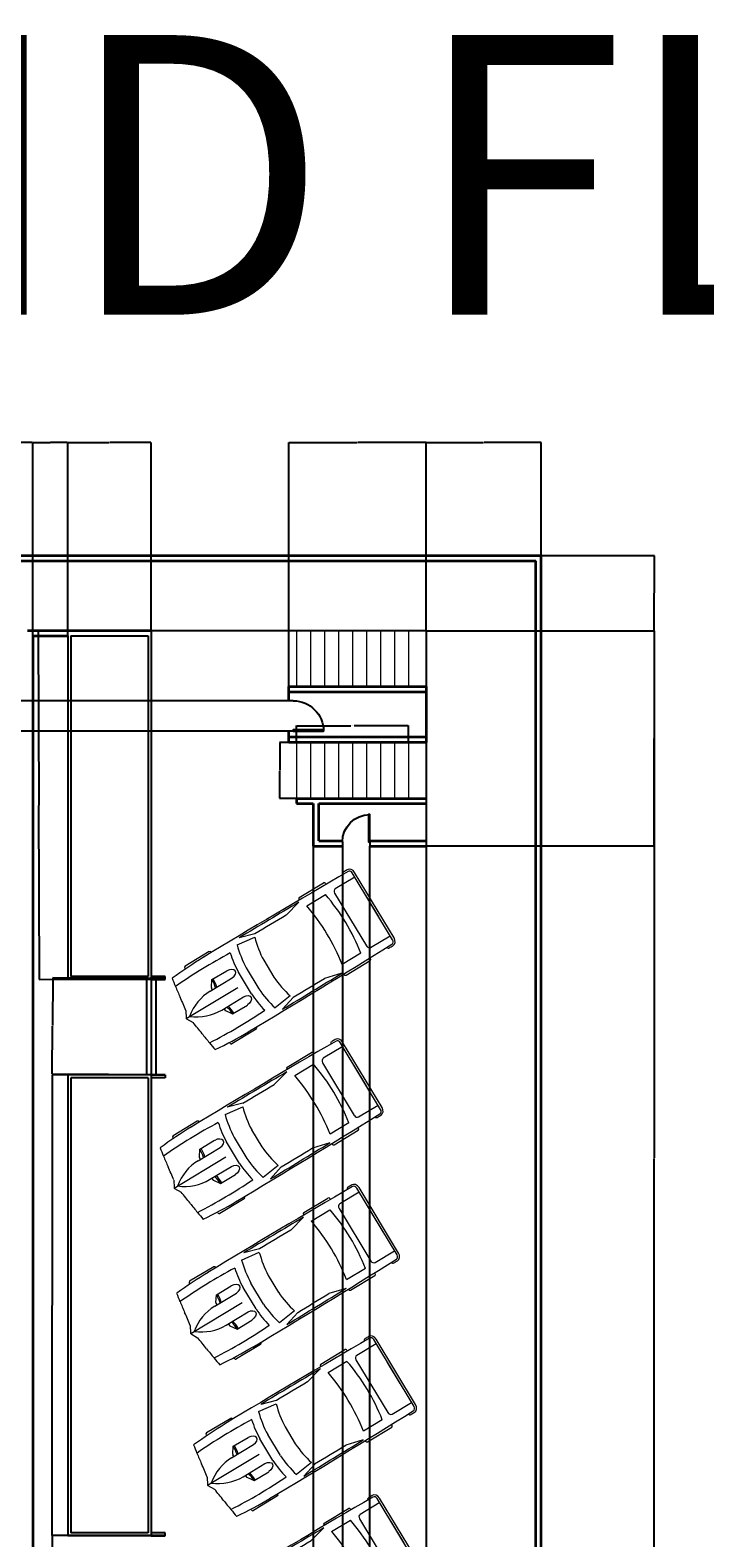
# Model space of a CAD drawing. Units: inches. Extents: x 1563 to 5866, y -225 to 2207.
# Tile 3 of 3: x 3624 to 4202, y 913 to 2207. Entities that reach past the tile are written whole.
import ezdxf

# ---------------------------------------------------------------- set-up
doc = ezdxf.new("R2010")
doc.units = ezdxf.units.IN
for name, color, linetype, lineweight in [('A-ANNO-DIMS', 2, 'Continuous', 18), ('A-ANNO-TEXT', 7, 'Continuous', 25), ('A-DOOR', 4, 'Continuous', 25), ('A-FLOR-STRS', 3, 'Continuous', 18), ('A-WALL', 7, 'Continuous', 35), ('C-PKNG', 8, 'Continuous', 25), ('C-PKNG-VEHI', 9, 'Continuous', 13), ('C-PROP', 2, 'Continuous', 35)]:
    doc.layers.add(name, color=color, linetype=linetype, lineweight=lineweight)
doc.styles.get("Standard").update_dxf_attribs({"font": 'arial.ttf'})
doc.dimstyles.get("Standard").update_dxf_attribs({"dimtxt": 0.18, "dimasz": 0.18, "dimexe": 0.18, "dimexo": 0.0625, "dimgap": 0.09, "dimtad": 0, "dimtih": 1, "dimtoh": 1, "dimdec": 4, "dimzin": 0, "dimdsep": 46, "dimtxsty": 'Standard', "dimcen": 0.09, "dimadec": 0, "dimazin": 0, "dimtfac": 1, "dimtdec": 4, "dimtofl": 0, "dimtmove": 0, "dimatfit": 3, "dimfxl": 1, "dimtolj": 1, "dimtzin": 0, "dimarcsym": 0})

# ---------------------------------------------------------------- blocks, each defined once
blk = doc.blocks.new('*U2')
for p, q in [((46.6, 38.9), (22.4, 38.9)), ((136.7, 38.9), (160.9, 38.9)), ((21.1, 37.4), (21.1, 36.8)), ((47.8, 37.4), (47.8, 37.4)), ((70, 31.5), (86.4, 29.4)), ((88, 31.9), (74.8, 35.9)), ((134.3, 35.6), (119.3, 31.8)), ((135.5, 37.1), (135.5, 37.4)), ((138.4, 29.4), (157.2, 29.4)), ((162.1, 37.4), (162.1, 36.8)), ((164.5, 26.4), (164.5, -26.4)), ((186.5, 29.4), (167, 29.4)), ((186.5, -33.5), (186.5, 33.5)), ((188.4, -32.8), (188.4, 32.8)), ((32.3, 11.6), (36.1, 17.2)), ((36.1, 17.2), (50.9, 17.2)), ((3.3, 6.1), (0.1, 0.4)), ((29.8, 9.5), (51.7, 9.5)), ((32.1, 9.5), (32.1, 11.2)), ((58.9, -10.8), (58.9, 10.8)), ((66.6, -10.5), (66.6, 10.5)), ((82.7, 8.5), (82.7, -8.5)), ((186.5, -10.5), (186.5, 10.5)), ((0, 0), (51.7, 0)), ((0.1, -0.4), (3.3, -6.1)), ((29.8, -9.5), (51.7, -9.5)), ((32.1, -9.5), (32.1, -11.2)), ((32.3, -11.6), (36.1, -17.2)), ((36.1, -17.2), (50.9, -17.2)), ((21.1, -37.4), (21.1, -36.8)), ((47.8, -37.4), (47.8, -37.4)), ((86.4, -29.4), (70, -31.5)), ((88, -31.9), (74.8, -35.9)), ((134.3, -35.6), (119.3, -31.8)), ((135.5, -37.1), (135.5, -37.4)), ((157.2, -29.4), (138.4, -29.4)), ((162.1, -37.4), (162.1, -36.8)), ((167, -29.4), (186.5, -29.4)), ((46.6, -38.9), (22.4, -38.9)), ((136.7, -38.9), (160.9, -38.9))]:
    blk.add_line(p, q)
for centre, major_axis, ratio, start_param, end_param in [((22.4, 37.4), (0, -1.48), 0.842304, 3.141593, 4.712389), ((46.6, 37.4), (0, 1.48), 0.842304, -1.570796, 0), ((136.7, 37.4), (0, -1.48), 0.842304, 3.141593, 4.712389), ((160.9, 37.4), (0, 1.48), 0.842304, -1.570796, 0), ((259.2, -27.5), (0, -305.3), 0.842304, 4.528606, 4.561838), ((266, -27.5), (0, 313.3), 0.842304, 1.367076, 1.39176), ((37.5, -594), (0, -623.3), 0.842304, 3.096046, 3.200911), ((41.2, -490.9), (0, 528.2), 0.842304, 0.00281, 0.075598), ((64.5, -10555.6), (0, 10593), 0.842304, -0.013397, 0.002797), ((134.4, 5.4), (0, -89.8), 0.842304, 4.449482, 4.652344), ((135.3, 5.4), (0, 81.8), 0.842304, 1.245306, 1.50788), ((64.5, -10555.6), (0, -10591.5), 0.842304, 3.133765, 3.140441), ((149.6, 2.8), (0, -79.6), 0.842304, 4.372215, 4.640744), ((95.8, -3666.4), (0, -3698.2), 0.842304, 3.134049, 3.144098), ((17.1, 0), (0, 147), 0.842304, 4.511394, 4.913384), ((35.9, 0), (0, 147), 0.842304, 4.511394, 4.913384), ((167, 26.4), (0, 2.96), 0.842304, 0, 1.570796), ((180.6, 35.8), (0, 2.22), 0.842304, -0.013017, 1.249894), ((64.5, -10556.4), (0, 10595.3), 0.842304, -0.013397, -0.013017), ((184, 32.8), (0, -5.25), 0.842304, 1.570796, 3.128196), ((184, 33.5), (0, -2.96), 0.842304, 1.570796, 3.128196), ((-204.5, 52.4), (0, -251), 0.842304, 1.385369, 1.434372), ((13, 17), (0, 27.4), 0.842304, 4.435146, 4.718221), ((14.2, 17), (0, 27.4), 0.842304, 4.435146, 4.718221), ((50.8, 13.3), (6.34, -0.36), 0.603834, -1.395552, 1.581315), ((0.6, 0), (0, -0.74), 0.842304, 4.131459, 5.293319), ((29.8, -46.7), (0, 56.2), 0.842304, 0, 0.590319), ((32.7, 11.2), (0, 0.74), 0.842304, 0.879714, 1.570796), ((-204.5, -52.4), (0, 251), 0.842304, -1.434372, -1.385369), ((29.8, 46.7), (0, 56.2), 0.842304, 2.551274, 3.141593), ((32.7, -11.2), (0, -0.74), 0.842304, 4.712389, 5.403472), ((13, -17), (0, -27.4), 0.842304, 1.564964, 1.848039), ((14.2, -17), (0, -27.4), 0.842304, 1.564964, 1.848039), ((134.4, -5.4), (0, -89.8), 0.842304, -1.510751, -1.307889), ((135.3, -5.4), (0, -81.8), 0.842304, -1.50788, -1.245306), ((149.6, -2.8), (0, -79.6), 0.842304, -1.499151, -1.230623), ((259.2, 27.5), (0, 305.3), 0.842304, 1.721348, 1.754579), ((266, 27.5), (0, 313.3), 0.842304, 1.749832, 1.774517), ((37.5, 594), (0, -623.3), 0.842304, -0.059319, 0.045547), ((41.2, 490.9), (0, -528.2), 0.842304, -0.075598, -0.00281), ((22.4, -37.4), (0, 1.48), 0.842304, 1.570796, 3.141593), ((64.5, 10555.6), (0, 10593), 0.842304, 3.138796, 3.15499), ((46.6, -37.4), (0, -1.48), 0.842304, 0, 1.570796), ((64.5, 10555.6), (0, -10591.5), 0.842304, 0.001152, 0.007828), ((95.8, 3666.4), (0, -3698.2), 0.842304, -0.002505, 0.007544), ((136.7, -37.4), (0, -1.48), 0.842304, -1.570796, 0), ((160.9, -37.4), (0, 1.48), 0.842304, 3.141593, 4.712389), ((167, -26.4), (0, -2.96), 0.842304, 4.712389, 6.283185), ((180.6, -35.8), (0, -2.22), 0.842304, -1.249894, 0.013017), ((64.5, 10556.4), (0, 10595.3), 0.842304, 3.15461, 3.15499), ((184, -32.8), (0, -5.25), 0.842304, 0.013397, 1.570796), ((184, -33.5), (0, 2.96), 0.842304, 3.15499, 4.712389)]:
    blk.add_ellipse(centre, major_axis=major_axis, ratio=ratio, start_param=start_param, end_param=end_param)
at = {"extrusion": (0, 0, -1)}
blk.add_ellipse((50.8, -13.3), major_axis=(6.34, 0.36), ratio=0.603834, start_param=-1.395552, end_param=1.581315, dxfattribs=at)
blk = doc.blocks.new('*U5')
for p, q in [((0, 0), (0, -6)), ((40, 0), (40, -6))]:
    blk.add_line(p, q)
blk.add_lwpolyline([(0, 0), (0, 40), (1.75, 40), (1.75, 0)], close=True)
blk.add_arc((0, 0), 40, 0, 90)
blk = doc.blocks.new('STAIR-FLIGHT-48IN')
for p, q in [((0, 48), (0, 0)), ((12, 48), (12, 0)), ((24, 48), (24, 0)), ((36, 48), (36, 0)), ((48, 48), (48, 0)), ((60, 48), (60, 0)), ((72, 48), (72, 0)), ((84, 48), (84, 0)), ((96, 48), (96, 0))]:
    blk.add_line(p, q)
blk = doc.blocks.new('*D16')
at = {"layer": 'A-ANNO-DIMS', "color": 0, "lineweight": -2, "transparency": 16777216}
for p, q in [((3852.2, 1595.9), (3852.2, 1610.4)), ((3852.4, 1610.2), (3898.8, 1610.2)), ((3948, 1610.2), (3901.6, 1610.2)), ((3948.2, 1595.9), (3948.2, 1610.4))]:
    blk.add_line(p, q, dxfattribs=at)
at = {"layer": 'A-ANNO-DIMS', "color": 0, "transparency": 16777216}
for points in [[(3852.4, 1610.2), (3852.4, 1610.2), (3852.2, 1610.2)], [(3948, 1610.2), (3948, 1610.2), (3948.2, 1610.2)]]:
    blk.add_solid(points, dxfattribs=at)
at = {"layer": 'Defpoints', "color": 0, "transparency": 16777216}
for p in [(3948.2, 1610.2), (3852.2, 1595.8), (3948.2, 1595.8)]:
    blk.add_point(p, dxfattribs=at)
at = {"layer": 'A-ANNO-DIMS', "color": 0, "transparency": 16777216, "insert": (3900.2, 1610.2), "char_height": 0.18, "attachment_point": 5}
blk.add_mtext('\\A1;STAIR FLIGHT 96 TYP.', dxfattribs=at)
blk = doc.blocks.new('*D17')
at = {"layer": 'A-ANNO-DIMS', "color": 0, "lineweight": -2, "transparency": 16777216}
for p, q in [((3852.1, 1595.8), (3837.6, 1595.8)), ((3837.8, 1595.6), (3837.8, 1572)), ((3837.8, 1548), (3837.8, 1571.6)), ((3852.1, 1547.8), (3837.6, 1547.8))]:
    blk.add_line(p, q, dxfattribs=at)
at = {"layer": 'A-ANNO-DIMS', "color": 0, "transparency": 16777216}
for points in [[(3837.8, 1595.6), (3837.8, 1595.6), (3837.8, 1595.8)], [(3837.8, 1548), (3837.8, 1548), (3837.8, 1547.8)]]:
    blk.add_solid(points, dxfattribs=at)
at = {"layer": 'Defpoints', "color": 0, "transparency": 16777216}
for p in [(3837.8, 1595.8), (3852.2, 1595.8), (3852.2, 1547.8)]:
    blk.add_point(p, dxfattribs=at)
at = {"layer": 'A-ANNO-DIMS', "color": 0, "transparency": 16777216, "insert": (3837.8, 1571.8), "char_height": 0.18, "attachment_point": 5}
blk.add_mtext('\\A1;48 TYP.', dxfattribs=at)
blk = doc.blocks.new('*D20')
at = {"layer": 'A-ANNO-DIMS', "color": 0, "lineweight": -2, "transparency": 16777216}
for p, q in [((3379.6, 1756.4), (3379.6, 1853.4)), ((3379.8, 1853.2), (3502.4, 1853.2)), ((3625.8, 1853.2), (3503.2, 1853.2)), ((3626, 1687.4), (3626, 1853.4))]:
    blk.add_line(p, q, dxfattribs=at)
at = {"layer": 'A-ANNO-DIMS', "color": 0, "transparency": 16777216}
for points in [[(3379.8, 1853.2), (3379.8, 1853.2), (3379.6, 1853.2)], [(3625.8, 1853.2), (3625.8, 1853.2), (3626, 1853.2)]]:
    blk.add_solid(points, dxfattribs=at)
at = {"layer": 'Defpoints', "color": 0, "transparency": 16777216}
for p in [(3626, 1853.2), (3379.6, 1756.3), (3626, 1687.3)]:
    blk.add_point(p, dxfattribs=at)
at = {"layer": 'A-ANNO-DIMS', "color": 0, "transparency": 16777216, "insert": (3502.8, 1853.2), "char_height": 0.18, "attachment_point": 5}
blk.add_mtext('\\A1;246.4', dxfattribs=at)
blk = doc.blocks.new('*D21')
at = {"layer": 'A-ANNO-DIMS', "color": 0, "lineweight": -2, "transparency": 16777216}
for p, q in [((3626, 1687.4), (3626, 1853.4)), ((3626.2, 1853.2), (3640.8, 1853.2)), ((3655.8, 1853.2), (3641.2, 1853.2)), ((3656, 1687.4), (3656, 1853.4))]:
    blk.add_line(p, q, dxfattribs=at)
at = {"layer": 'A-ANNO-DIMS', "color": 0, "transparency": 16777216}
for points in [[(3626.2, 1853.2), (3626.2, 1853.2), (3626, 1853.2)], [(3655.8, 1853.2), (3655.8, 1853.2), (3656, 1853.2)]]:
    blk.add_solid(points, dxfattribs=at)
at = {"layer": 'Defpoints', "color": 0, "transparency": 16777216}
for p in [(3656, 1853.2), (3626, 1687.3), (3656, 1687.3)]:
    blk.add_point(p, dxfattribs=at)
at = {"layer": 'A-ANNO-DIMS', "color": 0, "transparency": 16777216, "insert": (3641, 1853.2), "char_height": 0.18, "attachment_point": 5}
blk.add_mtext('\\A1;30', dxfattribs=at)
blk = doc.blocks.new('*D22')
at = {"layer": 'A-ANNO-DIMS', "color": 0, "lineweight": -2, "transparency": 16777216}
for p, q in [((3656, 1687.4), (3656, 1853.4)), ((3656.2, 1853.2), (3691.4, 1853.2)), ((3727.3, 1853.2), (3692.1, 1853.2)), ((3727.5, 1691.9), (3727.5, 1853.4))]:
    blk.add_line(p, q, dxfattribs=at)
at = {"layer": 'A-ANNO-DIMS', "color": 0, "transparency": 16777216}
for points in [[(3656.2, 1853.2), (3656.2, 1853.2), (3656, 1853.2)], [(3727.3, 1853.2), (3727.3, 1853.2), (3727.5, 1853.2)]]:
    blk.add_solid(points, dxfattribs=at)
at = {"layer": 'Defpoints', "color": 0, "transparency": 16777216}
for p in [(3727.5, 1853.2), (3656, 1687.3), (3727.5, 1691.8)]:
    blk.add_point(p, dxfattribs=at)
at = {"layer": 'A-ANNO-DIMS', "color": 0, "transparency": 16777216, "insert": (3691.7, 1853.2), "char_height": 0.18, "attachment_point": 5}
blk.add_mtext('\\A1;71.5', dxfattribs=at)
blk = doc.blocks.new('*D24')
at = {"layer": 'A-ANNO-DIMS', "color": 0, "lineweight": -2, "transparency": 16777216}
for p, q in [((3963.5, 1691.9), (3963.5, 1853.4)), ((3963.7, 1853.2), (4012.4, 1853.2)), ((4061.9, 1853.2), (4013.2, 1853.2)), ((4062.1, 1756.4), (4062.1, 1853.4))]:
    blk.add_line(p, q, dxfattribs=at)
at = {"layer": 'A-ANNO-DIMS', "color": 0, "transparency": 16777216}
for points in [[(3963.7, 1853.2), (3963.7, 1853.2), (3963.5, 1853.2)], [(4061.9, 1853.2), (4061.9, 1853.2), (4062.1, 1853.2)]]:
    blk.add_solid(points, dxfattribs=at)
at = {"layer": 'Defpoints', "color": 0, "transparency": 16777216}
for p in [(4062.1, 1853.2), (4062.1, 1756.3), (3963.5, 1691.8)]:
    blk.add_point(p, dxfattribs=at)
at = {"layer": 'A-ANNO-DIMS', "color": 0, "transparency": 16777216, "insert": (4012.8, 1853.2), "char_height": 0.18, "attachment_point": 5}
blk.add_mtext('\\A1;98.58', dxfattribs=at)
blk = doc.blocks.new('*D25')
at = {"layer": 'A-ANNO-DIMS', "color": 0, "lineweight": -2, "transparency": 16777216}
for p, q in [((4062.1, 1756.3), (4159.1, 1756.3)), ((4159, 1756.1), (4159, 1724.2)), ((4159, 1692), (4159, 1723.9)), ((3963.5, 1691.8), (4159.1, 1691.8))]:
    blk.add_line(p, q, dxfattribs=at)
at = {"layer": 'A-ANNO-DIMS', "color": 0, "transparency": 16777216}
for points in [[(4158.9, 1756.1), (4159, 1756.1), (4159, 1756.3)], [(4158.9, 1692), (4159, 1692), (4159, 1691.8)]]:
    blk.add_solid(points, dxfattribs=at)
at = {"layer": 'Defpoints', "color": 0, "transparency": 16777216}
for p in [(4062.1, 1756.3), (4159, 1756.3), (3963.5, 1691.8)]:
    blk.add_point(p, dxfattribs=at)
at = {"layer": 'A-ANNO-DIMS', "color": 0, "transparency": 16777216, "insert": (4159, 1724.1), "char_height": 0.18, "attachment_point": 5}
blk.add_mtext('\\A1;64.5', dxfattribs=at)
blk = doc.blocks.new('*D26')
at = {"layer": 'A-ANNO-DIMS', "color": 0, "lineweight": -2, "transparency": 16777216}
for p, q in [((3963.5, 1691.8), (4159.1, 1691.8)), ((4159, 1691.6), (4159, 1599.6)), ((4159, 1507.1), (4159, 1599.2)), ((3963.5, 1507), (4159.1, 1507))]:
    blk.add_line(p, q, dxfattribs=at)
at = {"layer": 'A-ANNO-DIMS', "color": 0, "transparency": 16777216}
for points in [[(4158.9, 1691.6), (4159, 1691.6), (4159, 1691.8)], [(4158.9, 1507.1), (4159, 1507.1), (4159, 1507)]]:
    blk.add_solid(points, dxfattribs=at)
at = {"layer": 'Defpoints', "color": 0, "transparency": 16777216}
for p in [(3963.5, 1691.8), (4159, 1691.8), (3963.5, 1507)]:
    blk.add_point(p, dxfattribs=at)
at = {"layer": 'A-ANNO-DIMS', "color": 0, "transparency": 16777216, "insert": (4159, 1599.4), "char_height": 0.18, "attachment_point": 5}
blk.add_mtext('\\A1;184.86', dxfattribs=at)
blk = doc.blocks.new('*D27')
at = {"layer": 'A-ANNO-DIMS', "color": 0, "lineweight": -2, "transparency": 16777216}
for p, q in [((3963.5, 1691.8), (4159.1, 1691.8)), ((4159, 1691.6), (4159, 1239.2)), ((4159, 786.4), (4159, 1238.8)), ((3963.5, 786.2), (4159.1, 786.2))]:
    blk.add_line(p, q, dxfattribs=at)
at = {"layer": 'A-ANNO-DIMS', "color": 0, "transparency": 16777216}
for points in [[(4158.9, 1691.6), (4159, 1691.6), (4159, 1691.8)], [(4158.9, 786.4), (4159, 786.4), (4159, 786.2)]]:
    blk.add_solid(points, dxfattribs=at)
at = {"layer": 'Defpoints', "color": 0, "transparency": 16777216}
for p in [(3963.5, 1691.8), (4159, 1691.8), (3963.5, 786.2)]:
    blk.add_point(p, dxfattribs=at)
at = {"layer": 'A-ANNO-DIMS', "color": 0, "transparency": 16777216, "insert": (4159, 1239), "char_height": 0.18, "attachment_point": 5}
blk.add_mtext('\\A1;905.6', dxfattribs=at)
blk = doc.blocks.new('*D39')
at = {"layer": 'A-ANNO-DIMS', "color": 0, "lineweight": -2, "transparency": 16777216}
for p, q in [((3727.4, 1691.8), (3630.4, 1691.5)), ((3630.6, 1691.3), (3631.1, 1542)), ((3631.6, 1392.3), (3631.1, 1541.6)), ((3728.5, 1392.5), (3631.5, 1392.1))]:
    blk.add_line(p, q, dxfattribs=at)
at = {"layer": 'A-ANNO-DIMS', "color": 0, "transparency": 16777216}
for points in [[(3630.6, 1691.3), (3630.6, 1691.3), (3630.6, 1691.5)], [(3631.7, 1392.3), (3631.6, 1392.3), (3631.6, 1392.1)]]:
    blk.add_solid(points, dxfattribs=at)
at = {"layer": 'Defpoints', "color": 0, "transparency": 16777216}
for p in [(3630.6, 1691.5), (3727.5, 1691.8), (3728.5, 1392.5)]:
    blk.add_point(p, dxfattribs=at)
at = {"layer": 'A-ANNO-DIMS', "color": 0, "transparency": 16777216, "insert": (3631.1, 1541.8), "char_height": 0.18, "attachment_point": 5}
blk.add_mtext('\\A1;299.36', dxfattribs=at)
blk = doc.blocks.new('*D40')
at = {"layer": 'A-ANNO-DIMS', "color": 0, "lineweight": -2, "transparency": 16777216}
for p, q in [((3643.3, 1393.8), (3642.9, 1352.8)), ((3740.1, 1393.1), (3643.1, 1393.9)), ((3642.6, 1311.4), (3642.9, 1352.4)), ((3739.4, 1310.5), (3642.4, 1311.2))]:
    blk.add_line(p, q, dxfattribs=at)
at = {"layer": 'A-ANNO-DIMS', "color": 0, "transparency": 16777216}
for points in [[(3643.2, 1393.8), (3643.3, 1393.8), (3643.3, 1393.9)], [(3642.6, 1311.4), (3642.6, 1311.4), (3642.6, 1311.2)]]:
    blk.add_solid(points, dxfattribs=at)
at = {"layer": 'Defpoints', "color": 0, "transparency": 16777216}
for p in [(3643.3, 1393.9), (3740.2, 1393.1), (3739.5, 1310.5)]:
    blk.add_point(p, dxfattribs=at)
at = {"layer": 'A-ANNO-DIMS', "color": 0, "transparency": 16777216, "insert": (3642.9, 1352.6), "char_height": 0.18, "attachment_point": 5}
blk.add_mtext('\\A1;82.7', dxfattribs=at)
blk = doc.blocks.new('*D41')
at = {"layer": 'A-ANNO-DIMS', "color": 0, "lineweight": -2, "transparency": 16777216}
for p, q in [((3739.4, 1310.5), (3642.4, 1310.5)), ((3642.6, 1310.3), (3642.6, 1112.9)), ((3642.6, 915.1), (3642.6, 1112.5)), ((3739.4, 915), (3642.4, 915))]:
    blk.add_line(p, q, dxfattribs=at)
at = {"layer": 'A-ANNO-DIMS', "color": 0, "transparency": 16777216}
for points in [[(3642.5, 1310.3), (3642.6, 1310.3), (3642.6, 1310.5)], [(3642.5, 915.1), (3642.6, 915.1), (3642.6, 915)]]:
    blk.add_solid(points, dxfattribs=at)
at = {"layer": 'Defpoints', "color": 0, "transparency": 16777216}
for p in [(3642.6, 1310.5), (3739.5, 1310.5), (3739.5, 915)]:
    blk.add_point(p, dxfattribs=at)
at = {"layer": 'A-ANNO-DIMS', "color": 0, "transparency": 16777216, "insert": (3642.6, 1112.7), "char_height": 0.18, "attachment_point": 5}
blk.add_mtext('\\A1;395.5', dxfattribs=at)
blk = doc.blocks.new('*D42')
at = {"layer": 'A-ANNO-DIMS', "color": 0, "lineweight": -2, "transparency": 16777216}
for p, q in [((3739.4, 915), (3642.4, 915)), ((3642.6, 914.8), (3642.6, 870.8)), ((3642.6, 826.6), (3642.6, 870.5)), ((3739.4, 826.4), (3642.4, 826.4))]:
    blk.add_line(p, q, dxfattribs=at)
at = {"layer": 'A-ANNO-DIMS', "color": 0, "transparency": 16777216}
for points in [[(3642.5, 914.8), (3642.6, 914.8), (3642.6, 915)], [(3642.5, 826.6), (3642.6, 826.6), (3642.6, 826.4)]]:
    blk.add_solid(points, dxfattribs=at)
at = {"layer": 'Defpoints', "color": 0, "transparency": 16777216}
for p in [(3642.6, 915), (3739.5, 915), (3739.5, 826.4)]:
    blk.add_point(p, dxfattribs=at)
at = {"layer": 'A-ANNO-DIMS', "color": 0, "transparency": 16777216, "insert": (3642.6, 870.7), "char_height": 0.18, "attachment_point": 5}
blk.add_mtext('\\A1;88.58', dxfattribs=at)
blk = doc.blocks.new('*D44')
at = {"layer": 'A-ANNO-DIMS', "color": 0, "lineweight": -2, "transparency": 16777216}
for p, q in [((3845.4, 1631.6), (2993.3, 1631.6)), ((2993.5, 1631.4), (2993.5, 1618.8)), ((2993.5, 1605.8), (2993.5, 1618.4)), ((3845.4, 1605.6), (2993.3, 1605.6))]:
    blk.add_line(p, q, dxfattribs=at)
at = {"layer": 'A-ANNO-DIMS', "color": 0, "transparency": 16777216}
for points in [[(2993.4, 1631.4), (2993.5, 1631.4), (2993.5, 1631.6)], [(2993.4, 1605.8), (2993.5, 1605.8), (2993.5, 1605.6)]]:
    blk.add_solid(points, dxfattribs=at)
at = {"layer": 'Defpoints', "color": 0, "transparency": 16777216}
for p in [(2993.5, 1631.6), (3845.5, 1631.6), (3845.5, 1605.6)]:
    blk.add_point(p, dxfattribs=at)
at = {"layer": 'A-ANNO-DIMS', "color": 0, "transparency": 16777216, "insert": (2993.5, 1618.6), "char_height": 0.18, "attachment_point": 5}
blk.add_mtext('\\A1;25.95', dxfattribs=at)
blk = doc.blocks.new('*D45')
at = {"layer": 'A-ANNO-DIMS', "color": 0, "lineweight": -2, "transparency": 16777216}
for p, q in [((3891.5, 1506.9), (3891.5, -225.3)), ((3914.9, 1506.9), (3914.9, -225.3)), ((3891.7, -225.1), (3902.8, -225.1)), ((3914.8, -225.1), (3903.6, -225.1))]:
    blk.add_line(p, q, dxfattribs=at)
at = {"layer": 'A-ANNO-DIMS', "color": 0, "transparency": 16777216}
for points in [[(3891.7, -225.1), (3891.7, -225.2), (3891.5, -225.1)], [(3914.8, -225.1), (3914.8, -225.2), (3914.9, -225.1)]]:
    blk.add_solid(points, dxfattribs=at)
at = {"layer": 'Defpoints', "color": 0, "transparency": 16777216}
for p in [(3891.5, 1507), (3914.9, 1507), (3914.9, -225.1)]:
    blk.add_point(p, dxfattribs=at)
at = {"layer": 'A-ANNO-DIMS', "color": 0, "transparency": 16777216, "insert": (3903.2, -225.1), "char_height": 0.18, "attachment_point": 5}
blk.add_mtext('\\A1;23.42', dxfattribs=at)
blk = doc.blocks.new('*D46')
at = {"layer": 'A-ANNO-DIMS', "color": 0, "lineweight": -2, "transparency": 16777216}
for p, q in [((3845.5, 1643.9), (3845.5, 1853.4)), ((3845.7, 1853.2), (3904.2, 1853.2)), ((3963.3, 1853.2), (3904.8, 1853.2)), ((3963.5, 1691.9), (3963.5, 1853.4))]:
    blk.add_line(p, q, dxfattribs=at)
at = {"layer": 'A-ANNO-DIMS', "color": 0, "transparency": 16777216}
for points in [[(3845.7, 1853.2), (3845.7, 1853.2), (3845.5, 1853.2)], [(3963.3, 1853.2), (3963.3, 1853.2), (3963.5, 1853.2)]]:
    blk.add_solid(points, dxfattribs=at)
at = {"layer": 'Defpoints', "color": 0, "transparency": 16777216}
for p in [(3963.5, 1853.2), (3963.5, 1691.8), (3845.5, 1643.8)]:
    blk.add_point(p, dxfattribs=at)
at = {"layer": 'A-ANNO-DIMS', "color": 0, "transparency": 16777216, "insert": (3904.5, 1853.2), "char_height": 0.18, "attachment_point": 5}
blk.add_mtext('\\A1;118', dxfattribs=at)
blk = doc.blocks.new('*D47')
at = {"layer": 'A-ANNO-DIMS', "color": 0, "lineweight": -2, "transparency": 16777216}
for p, q in [((3866.4, 1506.9), (3866.4, -225.3)), ((3891.5, 1506.9), (3891.5, -225.3)), ((3866.6, -225.1), (3878.5, -225.1)), ((3891.4, -225.1), (3879.4, -225.1))]:
    blk.add_line(p, q, dxfattribs=at)
at = {"layer": 'A-ANNO-DIMS', "color": 0, "transparency": 16777216}
for points in [[(3866.6, -225.1), (3866.6, -225.2), (3866.4, -225.1)], [(3891.4, -225.1), (3891.4, -225.2), (3891.5, -225.1)]]:
    blk.add_solid(points, dxfattribs=at)
at = {"layer": 'Defpoints', "color": 0, "transparency": 16777216}
for p in [(3866.4, 1507), (3891.5, 1507), (3891.5, -225.1)]:
    blk.add_point(p, dxfattribs=at)
at = {"layer": 'A-ANNO-DIMS', "color": 0, "transparency": 16777216, "insert": (3879, -225.1), "char_height": 0.18, "attachment_point": 5}
blk.add_mtext('\\A1;25.113', dxfattribs=at)
blk = doc.blocks.new('*D48')
at = {"layer": 'A-ANNO-DIMS', "color": 0, "lineweight": -2, "transparency": 16777216}
for p, q in [((3914.9, 1506.9), (3914.9, -225.3)), ((3963.5, 1506.9), (3963.5, -225.3)), ((3915.1, -225.1), (3938.8, -225.1)), ((3963.3, -225.1), (3939.6, -225.1))]:
    blk.add_line(p, q, dxfattribs=at)
at = {"layer": 'A-ANNO-DIMS', "color": 0, "transparency": 16777216}
for points in [[(3915.1, -225.1), (3915.1, -225.2), (3914.9, -225.1)], [(3963.3, -225.1), (3963.3, -225.2), (3963.5, -225.1)]]:
    blk.add_solid(points, dxfattribs=at)
at = {"layer": 'Defpoints', "color": 0, "transparency": 16777216}
for p in [(3914.9, 1507), (3963.5, 1507), (3963.5, -225.1)]:
    blk.add_point(p, dxfattribs=at)
at = {"layer": 'A-ANNO-DIMS', "color": 0, "transparency": 16777216, "insert": (3939.2, -225.1), "char_height": 0.18, "attachment_point": 5}
blk.add_mtext('\\A1;48.53', dxfattribs=at)

msp = doc.modelspace()

# ---------------------------------------------------------------- linework, layer by layer
at = {"layer": 'A-WALL'}
for p, q in [((3621.4794, 1691.8133), (3727.4794, 1691.8133)), ((3625.9794, 1687.3133), (3625.9794, 494.0374)), ((3625.9794, 1687.3133), (3655.9794, 1687.3133)), ((3845.4794, 1643.8133), (3963.4794, 1643.8133)), ((3845.4794, 1631.5836), (3845.4794, 1643.8133)), ((3963.4794, 1643.8133), (3963.4794, 1595.8133)), ((3845.4794, 1639.3133), (3963.4794, 1639.3133)), ((3845.4794, 1595.8133), (3845.4794, 1605.6311)), ((3963.4794, 1600.3133), (3845.4794, 1600.3133)), ((3963.4794, 1595.8133), (3845.4794, 1595.8133)), ((3852.1863, 1547.8133), (3963.4794, 1547.8133)), ((3852.1863, 1547.8133), (3852.1863, 1543.3133)), ((3852.1863, 1543.3133), (3866.4183, 1543.3133)), ((3866.4183, 1543.3133), (3866.4183, 1506.9516)), ((3871.4183, 1511.4516), (3871.4183, 1543.3133)), ((3871.4183, 1543.3133), (3963.4794, 1543.3133)), ((3866.4183, 1506.9516), (3891.5309, 1506.9516)), ((3866.4183, 1506.9516), (3871.4183, 1506.9516)), ((3871.4183, 1511.4516), (3891.5517, 1511.4516)), ((3913.9243, 1511.4516), (3963.4794, 1511.4516)), ((3914.9489, 1506.9516), (3963.4794, 1506.9516))]:
    msp.add_line(p, q, dxfattribs=at)
at = {"layer": 'C-PKNG'}
for p, q in [((3655.9794, 1687.3133), (3655.9794, 1392.3133)), ((3658.4794, 1687.3133), (3658.4794, 1394.8133)), ((3658.4794, 1687.3133), (3724.9794, 1687.3133)), ((3724.9794, 1687.3133), (3724.9794, 1394.8133)), ((3727.4794, 1691.8133), (3727.4794, 1392.3133)), ((3727.4794, 1691.8133), (3963.4794, 1691.8133)), ((3963.4794, 1691.8133), (3963.4794, 496.5374)), ((3727.4794, 1392.3133), (3655.9794, 1392.3133)), ((3724.9794, 1394.8133), (3658.4794, 1394.8133)), ((3723.3828, 1392.3133), (3723.3828, 1310.4515)), ((3739.4794, 1394.8133), (3727.4794, 1394.8133)), ((3727.4794, 1392.3133), (3739.4794, 1392.3133)), ((3727.4794, 1392.3133), (3727.4794, 1310.4515)), ((3731.5349, 1392.3133), (3731.5349, 1310.4515)), ((3739.4794, 1392.3133), (3739.4794, 1394.8133)), ((3727.4794, 1310.4515), (3655.9794, 1310.4515)), ((3655.9794, 1310.4515), (3655.9794, 914.9515)), ((3724.9794, 1307.9515), (3658.4794, 1307.9515)), ((3658.4794, 1307.9515), (3658.4794, 917.4515)), ((3724.9794, 1307.9515), (3724.9794, 917.4515)), ((3727.4794, 1310.4515), (3727.4794, 914.9515)), ((3727.4794, 1310.4515), (3739.4794, 1310.4515)), ((3739.4794, 1307.9515), (3727.4794, 1307.9515)), ((3739.4794, 1310.4515), (3739.4794, 1307.9515)), ((3727.4794, 914.9515), (3655.9794, 914.9515)), ((3724.9794, 917.4515), (3658.4794, 917.4515)), ((3739.4794, 917.4515), (3727.4794, 917.4515)), ((3727.4794, 914.9515), (3739.4794, 914.9515)), ((3739.4794, 914.9515), (3739.4794, 917.4515))]:
    msp.add_line(p, q, dxfattribs=at)
at = {"layer": 'C-PROP'}
for p, q in [((4057.5619, 446.938), (4057.5619, 1751.8133)), ((4062.0619, 444.2765), (4062.0619, 1756.3133))]:
    msp.add_line(p, q, dxfattribs=at)
for points in [[(3383.7523, 1756.3133), (3621.4794, 1756.3133), (4062.0619, 1756.3133)], [(3383.7523, 1751.8133), (3621.4794, 1751.8133), (4057.5619, 1751.8133)]]:
    msp.add_lwpolyline(points, dxfattribs=at)

# ---------------------------------------------------------------- block references
at = {"layer": 'A-DOOR', "xscale": -0.6488113845385353, "yscale": 0.6488113845385353, "zscale": 0.6488113845385353, "rotation": 270}
msp.add_blockref('*U5', (3849.3723, 1605.6311), dxfattribs=at)
at = {"layer": 'A-DOOR', "xscale": -0.5854489490070149, "yscale": 0.5854489490070149, "zscale": 0.5854489490070149}
msp.add_blockref('*U5', (3914.9489, 1510.4643), dxfattribs=at)
at = {"layer": 'A-FLOR-STRS'}
for p in [(3852.1863, 1643.8133), (3852.1863, 1547.8133)]:
    msp.add_blockref('STAIR-FLIGHT-48IN', p, dxfattribs=at)
at = {"layer": 'C-PKNG-VEHI', "rotation": 31.07575251048744}
for p in [(3757.5521, 1358.9065), (3747.234, 1213.3265), (3761.4008, 1088.4128), (3775.9101, 958.3032), (3778.9297, 821.878)]:
    msp.add_blockref('*U2', p, dxfattribs=at)

# ---------------------------------------------------------------- texts
at = {"layer": 'A-ANNO-TEXT'}
msp.add_text('SHOP GROUND FLOOR PLAN', height=240, dxfattribs=at).set_placement((1547.6082, 1963.0298))

# ---------------------------------------------------------------- dimensions: what is measured, and where the dimension line sits
at = {"layer": 'A-ANNO-DIMS'}
for base, p1, p2, override, picture, middle in [((3625.9794, 1853.2133), (3379.5737, 1756.3133), (3625.9794, 1687.3133), {"dimdec": 1, "dimlfac": 1, "dimrnd": 0, "dimzin": 0, "dimdsep": 46, "dimlunit": 2}, '*D20', (3502.7765, 1853.2133)), ((3655.9794, 1853.2133), (3625.9794, 1687.3133), (3655.9794, 1687.3133), {"dimdec": 0, "dimlfac": 1, "dimrnd": 0, "dimzin": 0, "dimdsep": 46, "dimlunit": 2}, '*D21', (3640.9794, 1853.2133)), ((3727.4794, 1853.2133), (3655.9794, 1687.3133), (3727.4794, 1691.8133), {"dimdec": 1, "dimlfac": 1, "dimrnd": 0, "dimzin": 0, "dimdsep": 46, "dimlunit": 2}, '*D22', (3691.7294, 1853.2133)), ((3963.4794, 1853.2133), (3845.4794, 1643.8133), (3963.4794, 1691.8133), {"dimdec": 0, "dimlfac": 1, "dimrnd": 0, "dimzin": 0, "dimdsep": 46, "dimlunit": 2}, '*D46', (3904.4794, 1853.2133)), ((4062.0619, 1853.2133), (3963.4794, 1691.8133), (4062.0619, 1756.3133), {"dimdec": 2, "dimlfac": 1, "dimrnd": 0, "dimzin": 0, "dimdsep": 46, "dimlunit": 2}, '*D24', (4012.7706, 1853.2133)), ((3891.5309, -225.1295), (3866.4183, 1506.9516), (3891.5309, 1506.9516), {"dimdec": 3, "dimlfac": 1, "dimrnd": 0, "dimzin": 0, "dimdsep": 46, "dimlunit": 2}, '*D47', (3878.9746, -225.1295)), ((3914.9489, -225.1295), (3891.5309, 1506.9516), (3914.9489, 1506.9516), {"dimdec": 2, "dimlfac": 1, "dimrnd": 0, "dimzin": 0, "dimdsep": 46, "dimlunit": 2}, '*D45', (3903.2399, -225.1295)), ((3963.4794, -225.1295), (3914.9489, 1506.9516), (3963.4794, 1506.9516), {"dimdec": 2, "dimlfac": 1, "dimrnd": 0, "dimzin": 0, "dimdsep": 46, "dimlunit": 2}, '*D48', (3939.2141, -225.1295))]:
    dim = msp.add_linear_dim(base=base, p1=p1, p2=p2, dimstyle='Standard', override=override, dxfattribs=at)
    dim.commit()
    dim.dimension.update_dxf_attribs({"geometry": picture, "text_midpoint": middle})
for base, p1, p2, angle, override, picture, middle in [((4158.9619, 1756.3133), (3963.4794, 1691.8133), (4062.0619, 1756.3133), 90, {"dimdec": 1, "dimlfac": 1, "dimrnd": 0, "dimzin": 0, "dimdsep": 46, "dimlunit": 2}, '*D25', (4158.9619, 1724.0633)), ((3630.58, 1691.4679), (3728.5462, 1392.453), (3727.4794, 1691.8133), 90.2041863, {"dimdec": 2, "dimlfac": 1, "dimrnd": 0, "dimzin": 0, "dimdsep": 46, "dimlunit": 2}, '*D39', (3631.1134, 1541.7878)), ((4158.9619, 1691.8133), (3963.4794, 1506.9516), (3963.4794, 1691.8133), 90, {"dimdec": 2, "dimlfac": 1, "dimrnd": 0, "dimzin": 0, "dimdsep": 46, "dimlunit": 2}, '*D26', (4158.9619, 1599.3824)), ((4158.9619, 1691.8133), (3963.4794, 786.2146), (3963.4794, 1691.8133), 90, {"dimdec": 1, "dimlfac": 1, "dimrnd": 0, "dimzin": 0, "dimdsep": 46, "dimlunit": 2}, '*D27', (4158.9619, 1239.0139)), ((2993.4766, 1631.5836), (3845.4794, 1605.6311), (3845.4794, 1631.5836), 90, {"dimdec": 2, "dimlfac": 1, "dimrnd": 0, "dimzin": 0, "dimdsep": 46, "dimlunit": 2}, '*D44', (2993.4766, 1618.6073)), ((3643.2579, 1393.9367), (3739.4794, 1310.4515), (3740.1547, 1393.1454), 89.5321149, {"dimdec": 1, "dimlfac": 1, "dimrnd": 0, "dimzin": 0, "dimdsep": 46, "dimlunit": 2}, '*D40', (3642.9203, 1352.5897)), ((3642.5794, 1310.4515), (3739.4794, 914.9515), (3739.4794, 1310.4515), 90, {"dimdec": 1, "dimlfac": 1, "dimrnd": 0, "dimzin": 0, "dimdsep": 46, "dimlunit": 2}, '*D41', (3642.5794, 1112.7015)), ((3642.5794, 914.9515), (3739.4794, 826.3734), (3739.4794, 914.9515), 90, {"dimdec": 2, "dimlfac": 1, "dimrnd": 0, "dimzin": 0, "dimdsep": 46, "dimlunit": 2}, '*D42', (3642.5794, 870.6624))]:
    dim = msp.add_linear_dim(base=base, p1=p1, p2=p2, angle=angle, dimstyle='Standard', override=override, dxfattribs=at)
    dim.commit()
    dim.dimension.update_dxf_attribs({"geometry": picture, "text_midpoint": middle})
dim = msp.add_linear_dim(base=(3948.1863, 1610.2133), p1=(3852.1863, 1595.8133), p2=(3948.1863, 1595.8133), text='STAIR FLIGHT <> TYP.', dimstyle='Standard', override={"dimdec": 0, "dimlfac": 1, "dimrnd": 0, "dimzin": 0, "dimdsep": 46, "dimlunit": 2}, dxfattribs=at)
dim.commit()
dim.dimension.update_dxf_attribs({"geometry": '*D16', "text_midpoint": (3900.1863, 1610.2133)})
dim = msp.add_linear_dim(base=(3837.7863, 1595.8133), p1=(3852.1863, 1547.8133), p2=(3852.1863, 1595.8133), angle=90, text='<> TYP.', dimstyle='Standard', override={"dimdec": 0, "dimlfac": 1, "dimrnd": 0, "dimzin": 0, "dimdsep": 46, "dimlunit": 2}, dxfattribs=at)
dim.commit()
dim.dimension.update_dxf_attribs({"geometry": '*D17', "text_midpoint": (3837.7863, 1571.8133)})

doc.saveas('drawing.dxf')
